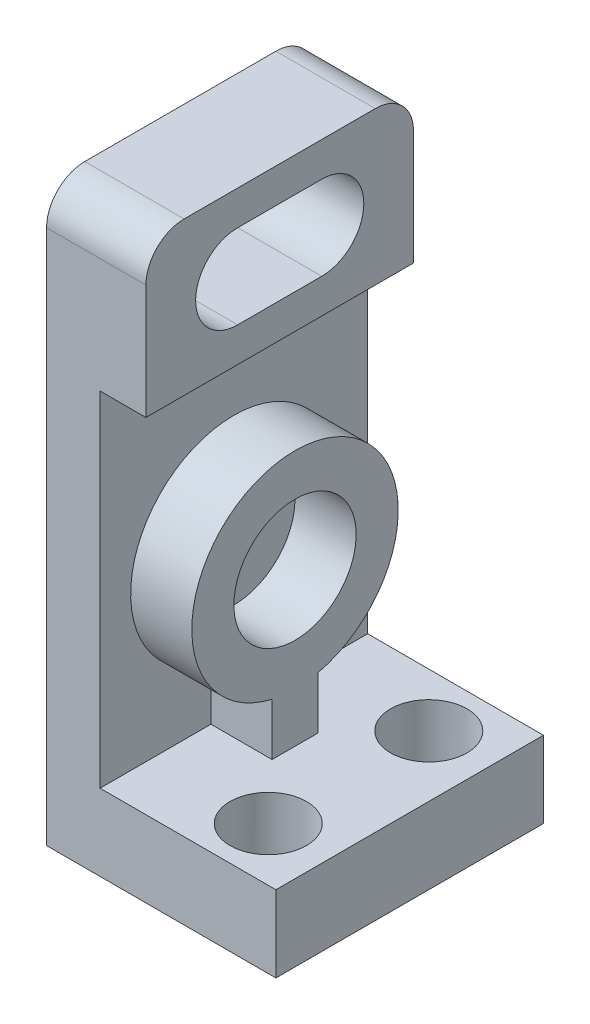
ISO-10303-21;
HEADER;
FILE_DESCRIPTION(('STEP AP214'),'2;1');
FILE_NAME('part.step','',(''),(''),'','','');
FILE_SCHEMA(('AUTOMOTIVE_DESIGN { 1 0 10303 214 1 1 1 1 }'));
ENDSEC;
DATA;
#1=APPLICATION_CONTEXT('core data for automotive mechanical design processes');
#2=APPLICATION_PROTOCOL_DEFINITION('international standard','automotive_design',2000,#1);
#3=PRODUCT_CONTEXT('',#1,'mechanical');
#4=PRODUCT('Part','Part','',(#3));
#5=PRODUCT_RELATED_PRODUCT_CATEGORY('part','',(#4));
#6=PRODUCT_DEFINITION_FORMATION('','',#4);
#7=PRODUCT_DEFINITION_CONTEXT('part definition',#1,'design');
#8=PRODUCT_DEFINITION('design','',#6,#7);
#9=PRODUCT_DEFINITION_SHAPE('','',#8);
#10=(LENGTH_UNIT() NAMED_UNIT(*) SI_UNIT(.MILLI.,.METRE.));
#11=(NAMED_UNIT(*) PLANE_ANGLE_UNIT() SI_UNIT($,.RADIAN.));
#12=(NAMED_UNIT(*) SI_UNIT($,.STERADIAN.) SOLID_ANGLE_UNIT());
#13=UNCERTAINTY_MEASURE_WITH_UNIT(LENGTH_MEASURE(1.E-05),#10,'distance_accuracy_value','');
#14=(GEOMETRIC_REPRESENTATION_CONTEXT(3) GLOBAL_UNCERTAINTY_ASSIGNED_CONTEXT((#13)) GLOBAL_UNIT_ASSIGNED_CONTEXT((#10,
#11,#12)) REPRESENTATION_CONTEXT('',''));
#15=CARTESIAN_POINT('',(0.,0.,0.));
#16=DIRECTION('',(0.,0.,1.));
#17=DIRECTION('',(1.,0.,0.));
#18=AXIS2_PLACEMENT_3D('',#15,#16,#17);
#19=CARTESIAN_POINT('',(7.,10.,-35.));
#20=DIRECTION('',(0.,1.,0.));
#21=DIRECTION('',(0.,0.,1.));
#22=AXIS2_PLACEMENT_3D('',#19,#20,#21);
#23=PLANE('',#22);
#24=CARTESIAN_POINT('',(22.,10.,-28.));
#25=DIRECTION('',(0.,1.,0.));
#26=DIRECTION('',(0.,0.,1.));
#27=AXIS2_PLACEMENT_3D('',#24,#25,#26);
#28=CIRCLE('',#27,5.);
#29=CARTESIAN_POINT('',(22.,10.,-23.));
#30=VERTEX_POINT('',#29);
#31=EDGE_CURVE('E230',#30,#30,#28,.T.);
#32=ORIENTED_EDGE('',*,*,#31,.F.);
#33=EDGE_LOOP('',(#32));
#34=FACE_BOUND('',#33,.T.);
#35=CARTESIAN_POINT('',(22.,10.,-7.));
#36=DIRECTION('',(0.,1.,0.));
#37=DIRECTION('',(0.,0.,1.));
#38=AXIS2_PLACEMENT_3D('',#35,#36,#37);
#39=CIRCLE('',#38,5.);
#40=CARTESIAN_POINT('',(22.,10.,-2.));
#41=VERTEX_POINT('',#40);
#42=EDGE_CURVE('E228',#41,#41,#39,.T.);
#43=ORIENTED_EDGE('',*,*,#42,.F.);
#44=EDGE_LOOP('',(#43));
#45=FACE_BOUND('',#44,.T.);
#46=DIRECTION('',(0.,0.,1.));
#47=VECTOR('',#46,1.);
#48=CARTESIAN_POINT('',(7.,10.,-35.));
#49=LINE('',#48,#47);
#50=CARTESIAN_POINT('',(7.,10.,-35.));
#51=VERTEX_POINT('',#50);
#52=CARTESIAN_POINT('',(7.,10.,-20.5));
#53=VERTEX_POINT('',#52);
#54=EDGE_CURVE('E296',#51,#53,#49,.T.);
#55=ORIENTED_EDGE('',*,*,#54,.T.);
#56=DIRECTION('',(-1.,0.,0.));
#57=VECTOR('',#56,1.);
#58=CARTESIAN_POINT('',(15.,10.,-20.5));
#59=LINE('',#58,#57);
#60=CARTESIAN_POINT('',(15.,10.,-20.5));
#61=VERTEX_POINT('',#60);
#62=EDGE_CURVE('E227',#61,#53,#59,.T.);
#63=ORIENTED_EDGE('',*,*,#62,.F.);
#64=DIRECTION('',(0.,0.,-1.));
#65=VECTOR('',#64,1.);
#66=CARTESIAN_POINT('',(15.,10.,-14.5));
#67=LINE('',#66,#65);
#68=CARTESIAN_POINT('',(15.,10.,-14.5));
#69=VERTEX_POINT('',#68);
#70=EDGE_CURVE('E204',#69,#61,#67,.T.);
#71=ORIENTED_EDGE('',*,*,#70,.F.);
#72=DIRECTION('',(-1.,0.,0.));
#73=VECTOR('',#72,1.);
#74=CARTESIAN_POINT('',(15.,10.,-14.5));
#75=LINE('',#74,#73);
#76=CARTESIAN_POINT('',(7.,10.,-14.5));
#77=VERTEX_POINT('',#76);
#78=EDGE_CURVE('E212',#69,#77,#75,.T.);
#79=ORIENTED_EDGE('',*,*,#78,.T.);
#80=CARTESIAN_POINT('',(7.,10.,0.));
#81=VERTEX_POINT('',#80);
#82=EDGE_CURVE('E298',#77,#81,#49,.T.);
#83=ORIENTED_EDGE('',*,*,#82,.T.);
#84=DIRECTION('',(-1.,0.,0.));
#85=VECTOR('',#84,1.);
#86=CARTESIAN_POINT('',(7.,10.,0.));
#87=LINE('',#86,#85);
#88=CARTESIAN_POINT('',(30.,10.,0.));
#89=VERTEX_POINT('',#88);
#90=EDGE_CURVE('E267',#89,#81,#87,.T.);
#91=ORIENTED_EDGE('',*,*,#90,.F.);
#92=DIRECTION('',(0.,0.,1.));
#93=VECTOR('',#92,1.);
#94=CARTESIAN_POINT('',(30.,10.,-35.));
#95=LINE('',#94,#93);
#96=CARTESIAN_POINT('',(30.,10.,-35.));
#97=VERTEX_POINT('',#96);
#98=EDGE_CURVE('E300',#97,#89,#95,.T.);
#99=ORIENTED_EDGE('',*,*,#98,.F.);
#100=DIRECTION('',(-1.,0.,0.));
#101=VECTOR('',#100,1.);
#102=CARTESIAN_POINT('',(7.,10.,-35.));
#103=LINE('',#102,#101);
#104=EDGE_CURVE('E247',#97,#51,#103,.T.);
#105=ORIENTED_EDGE('',*,*,#104,.T.);
#106=EDGE_LOOP('',(#55,#63,#71,#79,#83,#91,#99,#105));
#107=FACE_BOUND('',#106,.T.);
#108=ADVANCED_FACE('F41',(#34,#45,#107),#23,.T.);
#109=CARTESIAN_POINT('',(30.,0.,-35.));
#110=DIRECTION('',(0.,-1.,0.));
#111=DIRECTION('',(0.,0.,-1.));
#112=AXIS2_PLACEMENT_3D('',#109,#110,#111);
#113=PLANE('',#112);
#114=CARTESIAN_POINT('',(22.,0.,-28.));
#115=DIRECTION('',(0.,-1.,0.));
#116=DIRECTION('',(0.,0.,-1.));
#117=AXIS2_PLACEMENT_3D('',#114,#115,#116);
#118=CIRCLE('',#117,5.);
#119=CARTESIAN_POINT('',(22.,0.,-33.));
#120=VERTEX_POINT('',#119);
#121=EDGE_CURVE('E232',#120,#120,#118,.F.);
#122=ORIENTED_EDGE('',*,*,#121,.T.);
#123=EDGE_LOOP('',(#122));
#124=FACE_BOUND('',#123,.T.);
#125=CARTESIAN_POINT('',(22.,0.,-7.));
#126=DIRECTION('',(0.,-1.,0.));
#127=DIRECTION('',(0.,0.,-1.));
#128=AXIS2_PLACEMENT_3D('',#125,#126,#127);
#129=CIRCLE('',#128,5.);
#130=CARTESIAN_POINT('',(22.,0.,-12.));
#131=VERTEX_POINT('',#130);
#132=EDGE_CURVE('E240',#131,#131,#129,.F.);
#133=ORIENTED_EDGE('',*,*,#132,.T.);
#134=EDGE_LOOP('',(#133));
#135=FACE_BOUND('',#134,.T.);
#136=DIRECTION('',(1.,0.,0.));
#137=VECTOR('',#136,1.);
#138=CARTESIAN_POINT('',(30.,0.,0.));
#139=LINE('',#138,#137);
#140=CARTESIAN_POINT('',(0.,0.,0.));
#141=VERTEX_POINT('',#140);
#142=CARTESIAN_POINT('',(30.,0.,0.));
#143=VERTEX_POINT('',#142);
#144=EDGE_CURVE('E231',#141,#143,#139,.T.);
#145=ORIENTED_EDGE('',*,*,#144,.F.);
#146=DIRECTION('',(0.,0.,1.));
#147=VECTOR('',#146,1.);
#148=CARTESIAN_POINT('',(0.,0.,-35.));
#149=LINE('',#148,#147);
#150=CARTESIAN_POINT('',(0.,0.,-35.));
#151=VERTEX_POINT('',#150);
#152=EDGE_CURVE('E282',#151,#141,#149,.T.);
#153=ORIENTED_EDGE('',*,*,#152,.F.);
#154=DIRECTION('',(1.,0.,0.));
#155=VECTOR('',#154,1.);
#156=CARTESIAN_POINT('',(30.,0.,-35.));
#157=LINE('',#156,#155);
#158=CARTESIAN_POINT('',(30.,0.,-35.));
#159=VERTEX_POINT('',#158);
#160=EDGE_CURVE('E242',#151,#159,#157,.T.);
#161=ORIENTED_EDGE('',*,*,#160,.T.);
#162=DIRECTION('',(0.,0.,1.));
#163=VECTOR('',#162,1.);
#164=CARTESIAN_POINT('',(30.,0.,-35.));
#165=LINE('',#164,#163);
#166=EDGE_CURVE('E263',#159,#143,#165,.T.);
#167=ORIENTED_EDGE('',*,*,#166,.T.);
#168=EDGE_LOOP('',(#145,#153,#161,#167));
#169=FACE_BOUND('',#168,.T.);
#170=ADVANCED_FACE('F340',(#124,#135,#169),#113,.T.);
#171=CARTESIAN_POINT('',(0.,0.,-35.));
#172=DIRECTION('',(-1.,0.,0.));
#173=DIRECTION('',(0.,0.,1.));
#174=AXIS2_PLACEMENT_3D('',#171,#172,#173);
#175=PLANE('',#174);
#176=CARTESIAN_POINT('',(0.,65.,-23.));
#177=DIRECTION('',(-1.,0.,0.));
#178=DIRECTION('',(0.,0.,1.));
#179=AXIS2_PLACEMENT_3D('',#176,#177,#178);
#180=CIRCLE('',#179,5.5);
#181=CARTESIAN_POINT('',(0.,59.5,-23.));
#182=VERTEX_POINT('',#181);
#183=CARTESIAN_POINT('',(0.,70.5,-23.));
#184=VERTEX_POINT('',#183);
#185=EDGE_CURVE('E178',#182,#184,#180,.F.);
#186=ORIENTED_EDGE('',*,*,#185,.T.);
#187=DIRECTION('',(0.,0.,1.));
#188=VECTOR('',#187,1.);
#189=CARTESIAN_POINT('',(0.,70.5,-12.));
#190=LINE('',#189,#188);
#191=CARTESIAN_POINT('',(0.,70.5,-12.));
#192=VERTEX_POINT('',#191);
#193=EDGE_CURVE('E164',#184,#192,#190,.T.);
#194=ORIENTED_EDGE('',*,*,#193,.T.);
#195=CARTESIAN_POINT('',(0.,65.,-12.));
#196=DIRECTION('',(-1.,0.,0.));
#197=DIRECTION('',(0.,0.,1.));
#198=AXIS2_PLACEMENT_3D('',#195,#196,#197);
#199=CIRCLE('',#198,5.5);
#200=CARTESIAN_POINT('',(0.,59.5,-12.));
#201=VERTEX_POINT('',#200);
#202=EDGE_CURVE('E187',#192,#201,#199,.F.);
#203=ORIENTED_EDGE('',*,*,#202,.T.);
#204=DIRECTION('',(0.,0.,-1.));
#205=VECTOR('',#204,1.);
#206=CARTESIAN_POINT('',(0.,59.5,-23.));
#207=LINE('',#206,#205);
#208=EDGE_CURVE('E181',#201,#182,#207,.T.);
#209=ORIENTED_EDGE('',*,*,#208,.T.);
#210=EDGE_LOOP('',(#186,#194,#203,#209));
#211=FACE_BOUND('',#210,.T.);
#212=DIRECTION('',(0.,0.,1.));
#213=VECTOR('',#212,1.);
#214=CARTESIAN_POINT('',(0.,75.,-35.));
#215=LINE('',#214,#213);
#216=CARTESIAN_POINT('',(0.,75.,-30.));
#217=VERTEX_POINT('',#216);
#218=CARTESIAN_POINT('',(0.,75.,-5.));
#219=VERTEX_POINT('',#218);
#220=EDGE_CURVE('E288',#217,#219,#215,.T.);
#221=ORIENTED_EDGE('',*,*,#220,.F.);
#222=CARTESIAN_POINT('',(0.,70.,-30.));
#223=DIRECTION('',(-1.,0.,0.));
#224=DIRECTION('',(0.,0.,1.));
#225=AXIS2_PLACEMENT_3D('',#222,#223,#224);
#226=CIRCLE('',#225,5.);
#227=CARTESIAN_POINT('',(0.,70.,-35.));
#228=VERTEX_POINT('',#227);
#229=EDGE_CURVE('E315',#217,#228,#226,.T.);
#230=ORIENTED_EDGE('',*,*,#229,.T.);
#231=DIRECTION('',(0.,-1.,0.));
#232=VECTOR('',#231,1.);
#233=CARTESIAN_POINT('',(0.,0.,-35.));
#234=LINE('',#233,#232);
#235=EDGE_CURVE('E261',#228,#151,#234,.T.);
#236=ORIENTED_EDGE('',*,*,#235,.T.);
#237=ORIENTED_EDGE('',*,*,#152,.T.);
#238=DIRECTION('',(0.,-1.,0.));
#239=VECTOR('',#238,1.);
#240=CARTESIAN_POINT('',(0.,0.,0.));
#241=LINE('',#240,#239);
#242=CARTESIAN_POINT('',(0.,70.,0.));
#243=VERTEX_POINT('',#242);
#244=EDGE_CURVE('E248',#243,#141,#241,.T.);
#245=ORIENTED_EDGE('',*,*,#244,.F.);
#246=CARTESIAN_POINT('',(0.,70.,-5.));
#247=DIRECTION('',(-1.,0.,0.));
#248=DIRECTION('',(0.,0.,1.));
#249=AXIS2_PLACEMENT_3D('',#246,#247,#248);
#250=CIRCLE('',#249,5.);
#251=EDGE_CURVE('E309',#243,#219,#250,.T.);
#252=ORIENTED_EDGE('',*,*,#251,.T.);
#253=EDGE_LOOP('',(#221,#230,#236,#237,#245,#252));
#254=FACE_BOUND('',#253,.T.);
#255=ADVANCED_FACE('F182',(#211,#254),#175,.T.);
#256=CARTESIAN_POINT('',(0.,75.,-35.));
#257=DIRECTION('',(0.,1.,0.));
#258=DIRECTION('',(0.,0.,1.));
#259=AXIS2_PLACEMENT_3D('',#256,#257,#258);
#260=PLANE('',#259);
#261=DIRECTION('',(0.,0.,1.));
#262=VECTOR('',#261,1.);
#263=CARTESIAN_POINT('',(13.,75.,-35.));
#264=LINE('',#263,#262);
#265=CARTESIAN_POINT('',(13.,75.,-30.));
#266=VERTEX_POINT('',#265);
#267=CARTESIAN_POINT('',(13.,75.,-5.));
#268=VERTEX_POINT('',#267);
#269=EDGE_CURVE('E287',#266,#268,#264,.T.);
#270=ORIENTED_EDGE('',*,*,#269,.F.);
#271=DIRECTION('',(-1.,0.,0.));
#272=VECTOR('',#271,1.);
#273=CARTESIAN_POINT('',(0.,75.,-30.));
#274=LINE('',#273,#272);
#275=EDGE_CURVE('E307',#266,#217,#274,.T.);
#276=ORIENTED_EDGE('',*,*,#275,.T.);
#277=ORIENTED_EDGE('',*,*,#220,.T.);
#278=DIRECTION('',(-1.,0.,0.));
#279=VECTOR('',#278,1.);
#280=CARTESIAN_POINT('',(13.,75.,-5.));
#281=LINE('',#280,#279);
#282=EDGE_CURVE('E304',#219,#268,#281,.F.);
#283=ORIENTED_EDGE('',*,*,#282,.T.);
#284=EDGE_LOOP('',(#270,#276,#277,#283));
#285=FACE_BOUND('',#284,.T.);
#286=ADVANCED_FACE('F330',(#285),#260,.T.);
#287=CARTESIAN_POINT('',(13.,75.,-35.));
#288=DIRECTION('',(1.,0.,0.));
#289=DIRECTION('',(0.,1.,0.));
#290=AXIS2_PLACEMENT_3D('',#287,#288,#289);
#291=PLANE('',#290);
#292=CARTESIAN_POINT('',(13.,65.,-23.));
#293=DIRECTION('',(1.,0.,0.));
#294=DIRECTION('',(0.,1.,0.));
#295=AXIS2_PLACEMENT_3D('',#292,#293,#294);
#296=CIRCLE('',#295,5.5);
#297=CARTESIAN_POINT('',(13.,59.5,-23.));
#298=VERTEX_POINT('',#297);
#299=CARTESIAN_POINT('',(13.,70.5,-23.));
#300=VERTEX_POINT('',#299);
#301=EDGE_CURVE('E63',#298,#300,#296,.T.);
#302=ORIENTED_EDGE('',*,*,#301,.F.);
#303=DIRECTION('',(0.,0.,-1.));
#304=VECTOR('',#303,1.);
#305=CARTESIAN_POINT('',(13.,59.5,-23.));
#306=LINE('',#305,#304);
#307=CARTESIAN_POINT('',(13.,59.5,-12.));
#308=VERTEX_POINT('',#307);
#309=EDGE_CURVE('E176',#308,#298,#306,.T.);
#310=ORIENTED_EDGE('',*,*,#309,.F.);
#311=CARTESIAN_POINT('',(13.,65.,-12.));
#312=DIRECTION('',(1.,0.,0.));
#313=DIRECTION('',(0.,1.,0.));
#314=AXIS2_PLACEMENT_3D('',#311,#312,#313);
#315=CIRCLE('',#314,5.5);
#316=CARTESIAN_POINT('',(13.,70.5,-12.));
#317=VERTEX_POINT('',#316);
#318=EDGE_CURVE('E195',#317,#308,#315,.T.);
#319=ORIENTED_EDGE('',*,*,#318,.F.);
#320=DIRECTION('',(0.,0.,1.));
#321=VECTOR('',#320,1.);
#322=CARTESIAN_POINT('',(13.,70.5,-12.));
#323=LINE('',#322,#321);
#324=EDGE_CURVE('E183',#300,#317,#323,.T.);
#325=ORIENTED_EDGE('',*,*,#324,.F.);
#326=EDGE_LOOP('',(#302,#310,#319,#325));
#327=FACE_BOUND('',#326,.T.);
#328=DIRECTION('',(0.,1.,0.));
#329=VECTOR('',#328,1.);
#330=CARTESIAN_POINT('',(13.,75.,-35.));
#331=LINE('',#330,#329);
#332=CARTESIAN_POINT('',(13.,55.,-35.));
#333=VERTEX_POINT('',#332);
#334=CARTESIAN_POINT('',(13.,70.,-35.));
#335=VERTEX_POINT('',#334);
#336=EDGE_CURVE('E256',#333,#335,#331,.T.);
#337=ORIENTED_EDGE('',*,*,#336,.T.);
#338=CARTESIAN_POINT('',(13.,70.,-30.));
#339=DIRECTION('',(1.,0.,0.));
#340=DIRECTION('',(0.,1.,0.));
#341=AXIS2_PLACEMENT_3D('',#338,#339,#340);
#342=CIRCLE('',#341,5.);
#343=EDGE_CURVE('E47',#335,#266,#342,.T.);
#344=ORIENTED_EDGE('',*,*,#343,.T.);
#345=ORIENTED_EDGE('',*,*,#269,.T.);
#346=CARTESIAN_POINT('',(13.,70.,-5.));
#347=DIRECTION('',(1.,0.,0.));
#348=DIRECTION('',(0.,1.,0.));
#349=AXIS2_PLACEMENT_3D('',#346,#347,#348);
#350=CIRCLE('',#349,5.);
#351=CARTESIAN_POINT('',(13.,70.,0.));
#352=VERTEX_POINT('',#351);
#353=EDGE_CURVE('E316',#268,#352,#350,.T.);
#354=ORIENTED_EDGE('',*,*,#353,.T.);
#355=DIRECTION('',(0.,1.,0.));
#356=VECTOR('',#355,1.);
#357=CARTESIAN_POINT('',(13.,75.,0.));
#358=LINE('',#357,#356);
#359=CARTESIAN_POINT('',(13.,55.,0.));
#360=VERTEX_POINT('',#359);
#361=EDGE_CURVE('E279',#360,#352,#358,.T.);
#362=ORIENTED_EDGE('',*,*,#361,.F.);
#363=DIRECTION('',(0.,0.,1.));
#364=VECTOR('',#363,1.);
#365=CARTESIAN_POINT('',(13.,55.,-35.));
#366=LINE('',#365,#364);
#367=EDGE_CURVE('E295',#333,#360,#366,.T.);
#368=ORIENTED_EDGE('',*,*,#367,.F.);
#369=EDGE_LOOP('',(#337,#344,#345,#354,#362,#368));
#370=FACE_BOUND('',#369,.T.);
#371=ADVANCED_FACE('F319',(#327,#370),#291,.T.);
#372=CARTESIAN_POINT('',(13.,55.,-35.));
#373=DIRECTION('',(0.,-1.,0.));
#374=DIRECTION('',(0.,0.,-1.));
#375=AXIS2_PLACEMENT_3D('',#372,#373,#374);
#376=PLANE('',#375);
#377=DIRECTION('',(1.,0.,0.));
#378=VECTOR('',#377,1.);
#379=CARTESIAN_POINT('',(13.,55.,0.));
#380=LINE('',#379,#378);
#381=CARTESIAN_POINT('',(6.99999999999999,55.,0.));
#382=VERTEX_POINT('',#381);
#383=EDGE_CURVE('E274',#382,#360,#380,.T.);
#384=ORIENTED_EDGE('',*,*,#383,.F.);
#385=DIRECTION('',(0.,0.,1.));
#386=VECTOR('',#385,1.);
#387=CARTESIAN_POINT('',(6.99999999999999,55.,-35.));
#388=LINE('',#387,#386);
#389=CARTESIAN_POINT('',(6.99999999999999,55.,-35.));
#390=VERTEX_POINT('',#389);
#391=EDGE_CURVE('E294',#390,#382,#388,.T.);
#392=ORIENTED_EDGE('',*,*,#391,.F.);
#393=DIRECTION('',(1.,0.,0.));
#394=VECTOR('',#393,1.);
#395=CARTESIAN_POINT('',(13.,55.,-35.));
#396=LINE('',#395,#394);
#397=EDGE_CURVE('E254',#390,#333,#396,.T.);
#398=ORIENTED_EDGE('',*,*,#397,.T.);
#399=ORIENTED_EDGE('',*,*,#367,.T.);
#400=EDGE_LOOP('',(#384,#392,#398,#399));
#401=FACE_BOUND('',#400,.T.);
#402=ADVANCED_FACE('F351',(#401),#376,.T.);
#403=CARTESIAN_POINT('',(6.99999999999999,55.,-35.));
#404=DIRECTION('',(1.,0.,0.));
#405=DIRECTION('',(0.,1.,0.));
#406=AXIS2_PLACEMENT_3D('',#403,#404,#405);
#407=PLANE('',#406);
#408=CARTESIAN_POINT('',(7.,30.,-17.5));
#409=DIRECTION('',(1.,0.,0.));
#410=DIRECTION('',(0.,1.,0.));
#411=AXIS2_PLACEMENT_3D('',#408,#409,#410);
#412=CIRCLE('',#411,13.5);
#413=CARTESIAN_POINT('',(7.,16.8375534189118,-20.5));
#414=VERTEX_POINT('',#413);
#415=CARTESIAN_POINT('',(7.,16.8375534189118,-14.5));
#416=VERTEX_POINT('',#415);
#417=EDGE_CURVE('E216',#414,#416,#412,.T.);
#418=ORIENTED_EDGE('',*,*,#417,.F.);
#419=DIRECTION('',(0.,1.,0.));
#420=VECTOR('',#419,1.);
#421=CARTESIAN_POINT('',(7.,16.8375534189118,-20.5));
#422=LINE('',#421,#420);
#423=EDGE_CURVE('E201',#53,#414,#422,.T.);
#424=ORIENTED_EDGE('',*,*,#423,.F.);
#425=ORIENTED_EDGE('',*,*,#54,.F.);
#426=DIRECTION('',(0.,1.,0.));
#427=VECTOR('',#426,1.);
#428=CARTESIAN_POINT('',(6.99999999999999,55.,-35.));
#429=LINE('',#428,#427);
#430=EDGE_CURVE('E252',#51,#390,#429,.T.);
#431=ORIENTED_EDGE('',*,*,#430,.T.);
#432=ORIENTED_EDGE('',*,*,#391,.T.);
#433=DIRECTION('',(0.,1.,0.));
#434=VECTOR('',#433,1.);
#435=CARTESIAN_POINT('',(6.99999999999999,55.,0.));
#436=LINE('',#435,#434);
#437=EDGE_CURVE('E275',#81,#382,#436,.T.);
#438=ORIENTED_EDGE('',*,*,#437,.F.);
#439=ORIENTED_EDGE('',*,*,#82,.F.);
#440=DIRECTION('',(0.,-1.,0.));
#441=VECTOR('',#440,1.);
#442=CARTESIAN_POINT('',(7.,16.8375534189118,-14.5));
#443=LINE('',#442,#441);
#444=EDGE_CURVE('E208',#416,#77,#443,.T.);
#445=ORIENTED_EDGE('',*,*,#444,.F.);
#446=EDGE_LOOP('',(#418,#424,#425,#431,#432,#438,#439,#445));
#447=FACE_BOUND('',#446,.T.);
#448=ADVANCED_FACE('F358',(#447),#407,.T.);
#449=CARTESIAN_POINT('',(30.,10.,-35.));
#450=DIRECTION('',(1.,0.,0.));
#451=DIRECTION('',(0.,0.,-1.));
#452=AXIS2_PLACEMENT_3D('',#449,#450,#451);
#453=PLANE('',#452);
#454=DIRECTION('',(0.,1.,0.));
#455=VECTOR('',#454,1.);
#456=CARTESIAN_POINT('',(30.,10.,0.));
#457=LINE('',#456,#455);
#458=EDGE_CURVE('E266',#143,#89,#457,.T.);
#459=ORIENTED_EDGE('',*,*,#458,.F.);
#460=ORIENTED_EDGE('',*,*,#166,.F.);
#461=DIRECTION('',(0.,1.,0.));
#462=VECTOR('',#461,1.);
#463=CARTESIAN_POINT('',(30.,10.,-35.));
#464=LINE('',#463,#462);
#465=EDGE_CURVE('E245',#159,#97,#464,.T.);
#466=ORIENTED_EDGE('',*,*,#465,.T.);
#467=ORIENTED_EDGE('',*,*,#98,.T.);
#468=EDGE_LOOP('',(#459,#460,#466,#467));
#469=FACE_BOUND('',#468,.T.);
#470=ADVANCED_FACE('F361',(#469),#453,.T.);
#471=CARTESIAN_POINT('',(0.,0.,-35.));
#472=DIRECTION('',(0.,0.,-1.));
#473=DIRECTION('',(-1.,0.,0.));
#474=AXIS2_PLACEMENT_3D('',#471,#472,#473);
#475=PLANE('',#474);
#476=ORIENTED_EDGE('',*,*,#235,.F.);
#477=DIRECTION('',(-1.,0.,0.));
#478=VECTOR('',#477,1.);
#479=CARTESIAN_POINT('',(0.,70.,-35.));
#480=LINE('',#479,#478);
#481=EDGE_CURVE('E314',#228,#335,#480,.F.);
#482=ORIENTED_EDGE('',*,*,#481,.T.);
#483=ORIENTED_EDGE('',*,*,#336,.F.);
#484=ORIENTED_EDGE('',*,*,#397,.F.);
#485=ORIENTED_EDGE('',*,*,#430,.F.);
#486=ORIENTED_EDGE('',*,*,#104,.F.);
#487=ORIENTED_EDGE('',*,*,#465,.F.);
#488=ORIENTED_EDGE('',*,*,#160,.F.);
#489=EDGE_LOOP('',(#476,#482,#483,#484,#485,#486,#487,#488));
#490=FACE_BOUND('',#489,.T.);
#491=ADVANCED_FACE('F333',(#490),#475,.T.);
#492=CARTESIAN_POINT('',(0.,0.,0.));
#493=DIRECTION('',(0.,0.,-1.));
#494=DIRECTION('',(-1.,0.,0.));
#495=AXIS2_PLACEMENT_3D('',#492,#493,#494);
#496=PLANE('',#495);
#497=ORIENTED_EDGE('',*,*,#361,.T.);
#498=DIRECTION('',(-1.,0.,0.));
#499=VECTOR('',#498,1.);
#500=CARTESIAN_POINT('',(0.,70.,0.));
#501=LINE('',#500,#499);
#502=EDGE_CURVE('E11',#352,#243,#501,.T.);
#503=ORIENTED_EDGE('',*,*,#502,.T.);
#504=ORIENTED_EDGE('',*,*,#244,.T.);
#505=ORIENTED_EDGE('',*,*,#144,.T.);
#506=ORIENTED_EDGE('',*,*,#458,.T.);
#507=ORIENTED_EDGE('',*,*,#90,.T.);
#508=ORIENTED_EDGE('',*,*,#437,.T.);
#509=ORIENTED_EDGE('',*,*,#383,.T.);
#510=EDGE_LOOP('',(#497,#503,#504,#505,#506,#507,#508,#509));
#511=FACE_BOUND('',#510,.T.);
#512=ADVANCED_FACE('F342',(#511),#496,.F.);
#513=CARTESIAN_POINT('',(22.,-0.000999999999999265,-7.));
#514=DIRECTION('',(0.,1.,0.));
#515=DIRECTION('',(0.,0.,1.));
#516=AXIS2_PLACEMENT_3D('',#513,#514,#515);
#517=CYLINDRICAL_SURFACE('',#516,5.);
#518=ORIENTED_EDGE('',*,*,#132,.F.);
#519=EDGE_LOOP('',(#518));
#520=FACE_BOUND('',#519,.T.);
#521=ORIENTED_EDGE('',*,*,#42,.T.);
#522=EDGE_LOOP('',(#521));
#523=FACE_BOUND('',#522,.T.);
#524=ADVANCED_FACE('F423',(#520,#523),#517,.F.);
#525=CARTESIAN_POINT('',(22.,-0.000999999999999265,-28.));
#526=DIRECTION('',(0.,1.,0.));
#527=DIRECTION('',(0.,0.,1.));
#528=AXIS2_PLACEMENT_3D('',#525,#526,#527);
#529=CYLINDRICAL_SURFACE('',#528,5.);
#530=ORIENTED_EDGE('',*,*,#121,.F.);
#531=EDGE_LOOP('',(#530));
#532=FACE_BOUND('',#531,.T.);
#533=ORIENTED_EDGE('',*,*,#31,.T.);
#534=EDGE_LOOP('',(#533));
#535=FACE_BOUND('',#534,.T.);
#536=ADVANCED_FACE('F381',(#532,#535),#529,.F.);
#537=CARTESIAN_POINT('',(15.,30.,-17.5));
#538=DIRECTION('',(1.,0.,0.));
#539=DIRECTION('',(0.,1.,0.));
#540=AXIS2_PLACEMENT_3D('',#537,#538,#539);
#541=PLANE('',#540);
#542=ORIENTED_EDGE('',*,*,#70,.T.);
#543=DIRECTION('',(0.,1.,0.));
#544=VECTOR('',#543,1.);
#545=CARTESIAN_POINT('',(15.,16.8375534189118,-20.5));
#546=LINE('',#545,#544);
#547=CARTESIAN_POINT('',(15.,16.8375534189118,-20.5));
#548=VERTEX_POINT('',#547);
#549=EDGE_CURVE('E210',#61,#548,#546,.T.);
#550=ORIENTED_EDGE('',*,*,#549,.T.);
#551=CARTESIAN_POINT('',(15.,30.,-17.5));
#552=DIRECTION('',(1.,0.,0.));
#553=DIRECTION('',(0.,1.,0.));
#554=AXIS2_PLACEMENT_3D('',#551,#552,#553);
#555=CIRCLE('',#554,13.5);
#556=CARTESIAN_POINT('',(15.,16.8375534189118,-14.5));
#557=VERTEX_POINT('',#556);
#558=EDGE_CURVE('E209',#548,#557,#555,.T.);
#559=ORIENTED_EDGE('',*,*,#558,.T.);
#560=DIRECTION('',(0.,-1.,0.));
#561=VECTOR('',#560,1.);
#562=CARTESIAN_POINT('',(15.,16.8375534189118,-14.5));
#563=LINE('',#562,#561);
#564=EDGE_CURVE('E215',#557,#69,#563,.T.);
#565=ORIENTED_EDGE('',*,*,#564,.T.);
#566=EDGE_LOOP('',(#542,#550,#559,#565));
#567=FACE_BOUND('',#566,.T.);
#568=CARTESIAN_POINT('',(15.,30.,-17.5));
#569=DIRECTION('',(1.,0.,0.));
#570=DIRECTION('',(0.,1.,0.));
#571=AXIS2_PLACEMENT_3D('',#568,#569,#570);
#572=CIRCLE('',#571,8.);
#573=CARTESIAN_POINT('',(15.,38.,-17.5));
#574=VERTEX_POINT('',#573);
#575=EDGE_CURVE('E172',#574,#574,#572,.T.);
#576=ORIENTED_EDGE('',*,*,#575,.F.);
#577=EDGE_LOOP('',(#576));
#578=FACE_BOUND('',#577,.T.);
#579=ADVANCED_FACE('F378',(#567,#578),#541,.T.);
#580=CARTESIAN_POINT('',(15.,16.8375534189118,-20.5));
#581=DIRECTION('',(0.,0.,1.));
#582=DIRECTION('',(0.,-1.,0.));
#583=AXIS2_PLACEMENT_3D('',#580,#581,#582);
#584=PLANE('',#583);
#585=ORIENTED_EDGE('',*,*,#423,.T.);
#586=DIRECTION('',(-1.,0.,0.));
#587=VECTOR('',#586,1.);
#588=CARTESIAN_POINT('',(15.,16.8375534189118,-20.5));
#589=LINE('',#588,#587);
#590=EDGE_CURVE('E221',#548,#414,#589,.T.);
#591=ORIENTED_EDGE('',*,*,#590,.F.);
#592=ORIENTED_EDGE('',*,*,#549,.F.);
#593=ORIENTED_EDGE('',*,*,#62,.T.);
#594=EDGE_LOOP('',(#585,#591,#592,#593));
#595=FACE_BOUND('',#594,.T.);
#596=ADVANCED_FACE('F376',(#595),#584,.F.);
#597=CARTESIAN_POINT('',(15.,30.,-17.5));
#598=DIRECTION('',(-1.,0.,0.));
#599=DIRECTION('',(0.,-1.,0.));
#600=AXIS2_PLACEMENT_3D('',#597,#598,#599);
#601=CYLINDRICAL_SURFACE('',#600,13.5);
#602=ORIENTED_EDGE('',*,*,#417,.T.);
#603=DIRECTION('',(-1.,0.,0.));
#604=VECTOR('',#603,1.);
#605=CARTESIAN_POINT('',(15.,16.8375534189118,-14.5));
#606=LINE('',#605,#604);
#607=EDGE_CURVE('E222',#557,#416,#606,.T.);
#608=ORIENTED_EDGE('',*,*,#607,.F.);
#609=ORIENTED_EDGE('',*,*,#558,.F.);
#610=ORIENTED_EDGE('',*,*,#590,.T.);
#611=EDGE_LOOP('',(#602,#608,#609,#610));
#612=FACE_BOUND('',#611,.T.);
#613=ADVANCED_FACE('F373',(#612),#601,.T.);
#614=CARTESIAN_POINT('',(15.,16.8375534189118,-14.5));
#615=DIRECTION('',(0.,0.,-1.));
#616=DIRECTION('',(0.,1.,0.));
#617=AXIS2_PLACEMENT_3D('',#614,#615,#616);
#618=PLANE('',#617);
#619=ORIENTED_EDGE('',*,*,#444,.T.);
#620=ORIENTED_EDGE('',*,*,#78,.F.);
#621=ORIENTED_EDGE('',*,*,#564,.F.);
#622=ORIENTED_EDGE('',*,*,#607,.T.);
#623=EDGE_LOOP('',(#619,#620,#621,#622));
#624=FACE_BOUND('',#623,.T.);
#625=ADVANCED_FACE('F366',(#624),#618,.F.);
#626=CARTESIAN_POINT('',(15.,30.,-17.5));
#627=DIRECTION('',(-1.,0.,0.));
#628=DIRECTION('',(0.,-1.,0.));
#629=AXIS2_PLACEMENT_3D('',#626,#627,#628);
#630=CYLINDRICAL_SURFACE('',#629,8.);
#631=ORIENTED_EDGE('',*,*,#575,.T.);
#632=EDGE_LOOP('',(#631));
#633=FACE_BOUND('',#632,.T.);
#634=CARTESIAN_POINT('',(7.,30.,-17.5));
#635=DIRECTION('',(1.,0.,0.));
#636=DIRECTION('',(0.,1.,0.));
#637=AXIS2_PLACEMENT_3D('',#634,#635,#636);
#638=CIRCLE('',#637,8.);
#639=CARTESIAN_POINT('',(6.99999999999999,38.,-17.5));
#640=VERTEX_POINT('',#639);
#641=EDGE_CURVE('E285',#640,#640,#638,.F.);
#642=ORIENTED_EDGE('',*,*,#641,.T.);
#643=EDGE_LOOP('',(#642));
#644=FACE_BOUND('',#643,.T.);
#645=ADVANCED_FACE('F384',(#633,#644),#630,.F.);
#646=ORIENTED_EDGE('',*,*,#641,.F.);
#647=EDGE_LOOP('',(#646));
#648=FACE_BOUND('',#647,.T.);
#649=ADVANCED_FACE('F389',(#648),#407,.T.);
#650=CARTESIAN_POINT('',(0.,70.,-30.));
#651=DIRECTION('',(-1.,0.,0.));
#652=DIRECTION('',(0.,0.,1.));
#653=AXIS2_PLACEMENT_3D('',#650,#651,#652);
#654=CYLINDRICAL_SURFACE('',#653,5.);
#655=ORIENTED_EDGE('',*,*,#343,.F.);
#656=ORIENTED_EDGE('',*,*,#481,.F.);
#657=ORIENTED_EDGE('',*,*,#229,.F.);
#658=ORIENTED_EDGE('',*,*,#275,.F.);
#659=EDGE_LOOP('',(#655,#656,#657,#658));
#660=FACE_BOUND('',#659,.T.);
#661=ADVANCED_FACE('F329',(#660),#654,.T.);
#662=CARTESIAN_POINT('',(0.,70.,-5.));
#663=DIRECTION('',(1.,0.,0.));
#664=DIRECTION('',(0.,0.,-1.));
#665=AXIS2_PLACEMENT_3D('',#662,#663,#664);
#666=CYLINDRICAL_SURFACE('',#665,5.);
#667=ORIENTED_EDGE('',*,*,#353,.F.);
#668=ORIENTED_EDGE('',*,*,#282,.F.);
#669=ORIENTED_EDGE('',*,*,#251,.F.);
#670=ORIENTED_EDGE('',*,*,#502,.F.);
#671=EDGE_LOOP('',(#667,#668,#669,#670));
#672=FACE_BOUND('',#671,.T.);
#673=ADVANCED_FACE('F43',(#672),#666,.T.);
#674=CARTESIAN_POINT('',(-0.00100000000000447,65.,-23.));
#675=DIRECTION('',(1.,0.,0.));
#676=DIRECTION('',(0.,1.,0.));
#677=AXIS2_PLACEMENT_3D('',#674,#675,#676);
#678=CYLINDRICAL_SURFACE('',#677,5.5);
#679=DIRECTION('',(1.,0.,0.));
#680=VECTOR('',#679,1.);
#681=CARTESIAN_POINT('',(-0.00100000000000447,59.5,-23.));
#682=LINE('',#681,#680);
#683=EDGE_CURVE('E174',#182,#298,#682,.T.);
#684=ORIENTED_EDGE('',*,*,#683,.T.);
#685=ORIENTED_EDGE('',*,*,#301,.T.);
#686=DIRECTION('',(1.,0.,0.));
#687=VECTOR('',#686,1.);
#688=CARTESIAN_POINT('',(-0.0010000000000062,70.5,-23.));
#689=LINE('',#688,#687);
#690=EDGE_CURVE('E170',#184,#300,#689,.T.);
#691=ORIENTED_EDGE('',*,*,#690,.F.);
#692=ORIENTED_EDGE('',*,*,#185,.F.);
#693=EDGE_LOOP('',(#684,#685,#691,#692));
#694=FACE_BOUND('',#693,.T.);
#695=ADVANCED_FACE('F175',(#694),#678,.F.);
#696=CARTESIAN_POINT('',(-0.00100000000000447,59.5,-23.));
#697=DIRECTION('',(0.,-1.,0.));
#698=DIRECTION('',(1.,0.,0.));
#699=AXIS2_PLACEMENT_3D('',#696,#697,#698);
#700=PLANE('',#699);
#701=DIRECTION('',(1.,0.,0.));
#702=VECTOR('',#701,1.);
#703=CARTESIAN_POINT('',(-0.00100000000000447,59.5,-12.));
#704=LINE('',#703,#702);
#705=EDGE_CURVE('E196',#201,#308,#704,.T.);
#706=ORIENTED_EDGE('',*,*,#705,.T.);
#707=ORIENTED_EDGE('',*,*,#309,.T.);
#708=ORIENTED_EDGE('',*,*,#683,.F.);
#709=ORIENTED_EDGE('',*,*,#208,.F.);
#710=EDGE_LOOP('',(#706,#707,#708,#709));
#711=FACE_BOUND('',#710,.T.);
#712=ADVANCED_FACE('F539',(#711),#700,.F.);
#713=CARTESIAN_POINT('',(-0.00100000000000447,65.,-12.));
#714=DIRECTION('',(1.,0.,0.));
#715=DIRECTION('',(0.,1.,0.));
#716=AXIS2_PLACEMENT_3D('',#713,#714,#715);
#717=CYLINDRICAL_SURFACE('',#716,5.5);
#718=DIRECTION('',(1.,0.,0.));
#719=VECTOR('',#718,1.);
#720=CARTESIAN_POINT('',(-0.0010000000000062,70.5,-12.));
#721=LINE('',#720,#719);
#722=EDGE_CURVE('E57',#192,#317,#721,.T.);
#723=ORIENTED_EDGE('',*,*,#722,.T.);
#724=ORIENTED_EDGE('',*,*,#318,.T.);
#725=ORIENTED_EDGE('',*,*,#705,.F.);
#726=ORIENTED_EDGE('',*,*,#202,.F.);
#727=EDGE_LOOP('',(#723,#724,#725,#726));
#728=FACE_BOUND('',#727,.T.);
#729=ADVANCED_FACE('F548',(#728),#717,.F.);
#730=CARTESIAN_POINT('',(-0.0010000000000062,70.5,-12.));
#731=DIRECTION('',(0.,1.,0.));
#732=DIRECTION('',(-1.,0.,0.));
#733=AXIS2_PLACEMENT_3D('',#730,#731,#732);
#734=PLANE('',#733);
#735=ORIENTED_EDGE('',*,*,#690,.T.);
#736=ORIENTED_EDGE('',*,*,#324,.T.);
#737=ORIENTED_EDGE('',*,*,#722,.F.);
#738=ORIENTED_EDGE('',*,*,#193,.F.);
#739=EDGE_LOOP('',(#735,#736,#737,#738));
#740=FACE_BOUND('',#739,.T.);
#741=ADVANCED_FACE('F167',(#740),#734,.F.);
#742=CLOSED_SHELL('',(#108,#170,#255,#286,#371,#402,#448,#470,#491,#512,#524,#536,#579,#596,
#613,#625,#645,#649,#661,#673,#695,#712,#729,#741));
#743=MANIFOLD_SOLID_BREP('B2',#742);
#744=ADVANCED_BREP_SHAPE_REPRESENTATION('',(#18,#743),#14);
#745=SHAPE_DEFINITION_REPRESENTATION(#9,#744);
ENDSEC;
END-ISO-10303-21;
